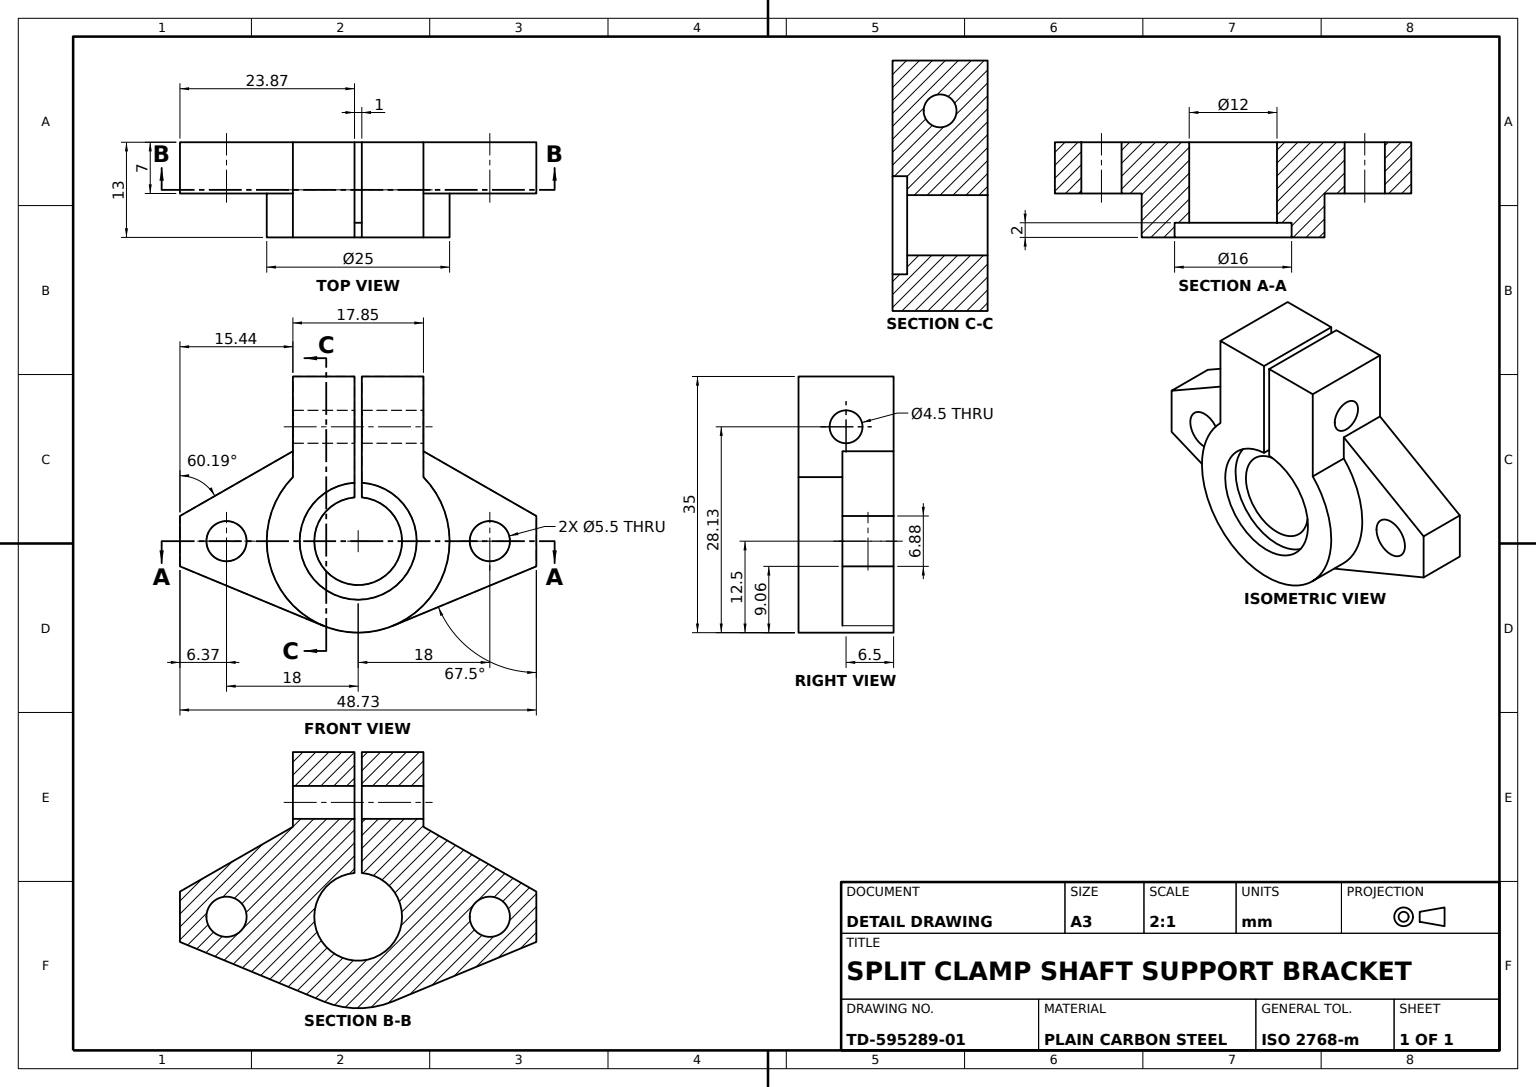
SolidWorks part; units mm, degrees
material "Plain Carbon Steel"
ref_plane "Front Plane" through (0, 0, 0) normal (0, 0, 1) x (1, 0, 0)
ref_plane "Top Plane" through (0, 0, 0) normal (0, 1, 0) x (1, 0, 0)
ref_plane "Right Plane" through (0, 0, 0) normal (1, 0, 0) x (0, 0, -1)
sketch "Clamp Ring Sketch" plane through (0, 0, 0) normal (0, 0, 1) x (1, 0, 0)
  line L0 (0, 0) -> (0, 12.5) construction
  line L1 (0, 0) -> (0, -12.5) construction
  circle A1 centre (0, 0) radius 12.5
  dimension "D2" = 25
extrude "Clamp Ring Ø25" add sketch "Clamp Ring Sketch" along normal blind 13
ref_plane "Plane1" through (0, 0, 0) normal (0, 0, 1) x (1, 0, 0)
sketch "Clamp Block Sketch" plane through (0, 0, 0) normal (0, 0, 1) x (1, 0, 0)
  line L0 (0, 0) -> (0, 22.5) construction
  line L1 (-8.925, 22.5) -> (8.925, 22.5)
  line L3 (-8.925, 22.5) -> (-8.925, 8.7518)
  line L4 (8.925, 22.5) -> (8.925, 8.7518)
  arc A6 (8.925, 8.7518) -> (-8.925, 8.7518) centre (0, 0) ccw
  dimension "D3" = 17.85
  dimension "D4" = 13.7482
  dimension "D1" = 25
  dimension "D2" = 13.7482
extrude "Clamp Block" add sketch "Clamp Block Sketch" along normal blind 13
sketch "Bore Sketch" plane through (0, 0, 13) normal (0, 0, 1) x (1, 0, 0)
  circle A0 centre (0, 0) radius 6
  dimension "D1" = 12
extrude "Bore Ø12" cut sketch "Bore Sketch" against normal blind 13
sketch "Counterbore Sketch" plane through (0, 0, 13) normal (0, 0, 1) x (1, 0, 0)
  circle A0 centre (0, 0) radius 8
  dimension "D1" = 16
extrude "Counterbore Ø16x2" cut sketch "Counterbore Sketch" against normal blind 2
ref_plane "Plane2" through (0, 0, 0) normal (0, 0, 1) x (1, 0, 0)
sketch "Mounting Flange Sketch" plane through (0, 0, 0) normal (0, 0, 1) x (1, 0, 0)
  line L0 (0, 0) -> (-24.3661, 0) construction
  line L1 (0, 0) -> (24.3592, 0) construction
  line L2 (0, 0) -> (-18, 0) construction
  line L3 (0, 0) -> (18, 0) construction
  line L4 (0, -12.5) -> (-31.6729, -12.5) construction
  line L5 (-24.3661, 3.44) -> (-24.3661, -3.4371)
  line L7 (-4.7835, -11.5485) -> (-24.3661, -3.4371)
  line L9 (-8.925, 22.5) -> (-8.925, 8.7518) construction
  line L12 (-8.925, 12.286) -> (-8.925, 8.7518)
  line L13 (24.3592, 3.44) -> (24.3592, -3.44)
  line L15 (-24.3661, 3.44) -> (-8.925, 12.286)
  line L16 (0, -12.5) -> (30.6609, -12.5) construction
  line L17 (4.7835, -11.5485) -> (24.3592, -3.44)
  line L18 (8.925, 12.286) -> (8.925, 8.7518)
  line L20 (24.3592, 3.44) -> (8.925, 12.286)
  circle A0 centre (-18, 0) radius 2.75
  circle A1 centre (18, 0) radius 2.75
  arc A2 (-8.925, 8.7518) -> (8.925, 8.7518) centre (0, 0) ccw construction
  arc A6 (-8.925, 8.7518) -> (8.925, 8.7518) centre (0, 0) ccw
  point P26 (-8.925, 10.9496)
  dimension "D1" = 5.5
  dimension "D2" = 5.5
  dimension "D6" = 24.3661
  dimension "D7" = 23.4496
  dimension "D3" = 18
  dimension "D4" = 18
  dimension "D5" = 22.5
  dimension "D8" = 12.286
  dimension "D9" = 22.5
  dimension "D10" = 24.3592
  dimension "D11" = 12.286
  dimension "D12" = 3.44
  dimension "D13" = 3.44
extrude "Mounting Flange 2xØ5.5" add sketch "Mounting Flange Sketch" along normal blind 7 contours A6 L12 L15 L5 L7 A0 | A6 L17 L13 L20 L18 A1
ref_plane "Plane3" through (0, 0, 13) normal (0, 0, 1) x (1, 0, 0)
sketch "Split Slot Sketch" plane through (0, 0, 13) normal (0, 0, 1) x (1, 0, 0)
  line L0 (0, 6) -> (0, 22.5) construction
  line L1 (8.925, 22.5) -> (-8.925, 22.5) construction
  line L2 (0.5, 5.9791) -> (0.5, 22.5)
  line L3 (-0.5, 5.9791) -> (-0.5, 22.5)
  line L4 (-0.5, 22.5) -> (0.5, 22.5)
  line L6 (-0.5, 0) -> (-0.5, 22.5) construction
  line L7 (0.5, 0) -> (0.5, 22.5) construction
  line L8 (0, 0) -> (0, 22.5) construction
  arc A1 (0.5, 5.9791) -> (-0.5, 5.9791) centre (0, 0) ccw
  dimension "D3" = 12
  dimension "D1" = 0.5
  dimension "D2" = 0.5
extrude "Clamp Split Slot" cut sketch "Split Slot Sketch" against normal through all
sketch "Clamp Screw Hole Sketch" plane through (8.925, 0, 0) normal (1, 0, 0) x (0, 0, -1)
  line L0 (-6.5, 22.5) -> (-6.5, 8.7518) construction
  line L2 (-6.5, 8.7518) -> (-13, 8.7518) construction
  line L3 (-13, 22.5) -> (0, 22.5) construction
  circle A0 centre (-6.5, 15.6259) radius 2.25
  dimension "D1" = 4.5
extrude "Clamp Screw Hole Ø4.5" cut sketch "Clamp Screw Hole Sketch" against normal blind 20
